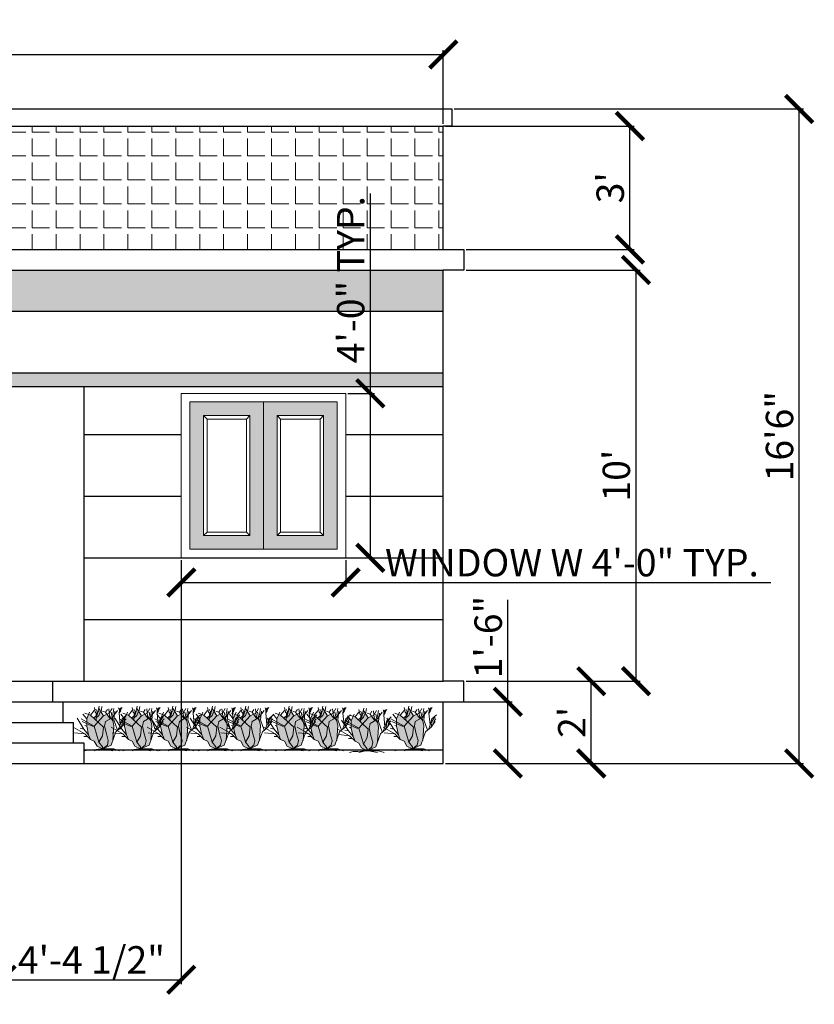
# Model space of a CAD drawing. Units: inches. Extents: x 21865 to 22885, y 36660 to 37408.
# Tile 6 of 6: x 22653 to 22885, y 36873 to 37161. Entities that reach past the tile are written whole.
import ezdxf

# ---------------------------------------------------------------- set-up
doc = ezdxf.new("R2010")
doc.units = ezdxf.units.IN
for name, color, linetype, lineweight in [('A-ANNO-DIMS', 2, 'Continuous', 18), ('A-ELEV', 7, 'Continuous', 30), ('A-ELEV-GLAZ', 4, 'Continuous', 18), ('A-ELEV-ROOF', 7, 'Continuous', 25), ('A-ELEV-ROOF-PATT', 8, 'Continuous', 13), ('L-PLNT', 94, 'Continuous', 13)]:
    doc.layers.add(name, color=color, linetype=linetype, lineweight=lineweight)
for name, color, linetype, lineweight, true_color in [('A-ELEV-TRIM-PATT', 51, 'Continuous', 13, 0xf7f281), ('A-ELEV-WALL-PATT', 251, 'Continuous', 13, 0x636466), ('L-PLNT-PATT', 114, 'Continuous', 13, 0x139b48)]:
    doc.layers.add(name, color=color, linetype=linetype, lineweight=lineweight, true_color=true_color)
doc.styles.get("Standard").update_dxf_attribs({"font": 'arial.ttf'})
doc.dimstyles.new('ISO-25', dxfattribs={"dimtxt": 8, "dimasz": 8, "dimexe": 1.25, "dimexo": 0.625, "dimtad": 1, "dimlunit": 3, "dimtxsty": 'Standard', "dimblk": 'ARCHTICK', "dimcen": 2.5, "dimclrd": 4, "dimclre": 5, "dimclrt": 1, "dimadec": 0, "dimazin": 0, "dimtfac": 1, "dimtmove": 0, "dimatfit": 3, "dimfxl": 1, "dimarcsym": 0})

# ---------------------------------------------------------------- blocks, each defined once
blk = doc.blocks.new('*U12')
for p, q in [((-14.88, 18.24), (-12.96, 20.64)), ((-12.471, 19.775), (-12.898, 22.044)), ((-11.28, 19.619), (-12.104, 21.184)), ((-11.921, 18.836), (-10.64, 20.401)), ((-11.433, 18.289), (-10.457, 22.749)), ((-8.16, 17.76), (-10.56, 21.6)), ((-9.48, 19.775), (-8.992, 22.592)), ((-7.2, 19.68), (-8.64, 20.16)), ((-7.2, 19.68), (-6.24, 21.12)), ((-5.086, 17.741), (-5.513, 21.34)), ((-5.28, 19.2), (-3.84, 21.6)), ((-3.84, 16.8), (-0.96, 20.64)), ((-3.377, 18.602), (-2.888, 21.575)), ((-2.88, 15.84), (-2.4, 20.16)), ((-0.508, 21.888), (-0.081, 20.558)), ((-0.203, 19.149), (0.102, 21.34)), ((-0.142, 19.384), (0.59, 20.401)), ((-0.02, 20.01), (0.896, 21.105)), ((0.041, 20.714), (1.384, 22.044)), ((0.102, 21.34), (0.835, 21.888)), ((-18.24, 11.04), (-21.755, 16.655)), ((-12.96, 12.48), (-19.68, 16.32)), ((-16.8, 16.32), (-18.72, 18.72)), ((-14.88, 18.24), (-17.76, 19.2)), ((-16.8, 16.32), (-15.36, 19.68)), ((-16.8, 12.48), (-16.8, 16.32)), ((-8.16, 12), (-14.88, 18.24)), ((-13.325, 16.724), (-11.433, 18.289)), ((-12.96, 12.48), (-8.16, 17.76)), ((-11.677, 19.071), (-12.471, 19.775)), ((-12.043, 15.628), (-11.921, 18.836)), ((-11.982, 16.802), (-10.579, 18.054)), ((-10.579, 18.054), (-9.846, 19.697)), ((-8.16, 17.76), (-5.28, 19.2)), ((-4.8, 16.32), (-7.2, 19.68)), ((-7.2, 14.88), (-3.84, 16.8)), ((-3.377, 15.315), (-5.086, 17.819)), ((-2.88, 12.96), (-4.32, 19.68)), ((-2.766, 16.802), (-3.377, 18.602)), ((-0.96, 10.56), (-2.88, 15.84)), ((0.346, 13.203), (-0.203, 19.149)), ((0.346, 13.203), (1.323, 16.254)), ((0.96, 12), (1.44, 15.36)), ((1.323, 16.254), (3.642, 18.289)), ((1.44, 15.36), (2.88, 17.28)), ((1.92, 13.44), (2.4, 15.36)), ((2.4, 15.36), (3.36, 16.32)), ((-17.76, 8.64), (-23.663, 11.961)), ((-18.24, 11.04), (-20.16, 11.52)), ((-13.92, 12.48), (-19.2, 14.88)), ((-15.84, 8.16), (-18.24, 11.04)), ((-16.8, 12.48), (-17.76, 12.96)), ((-15.84, 8.16), (-16.8, 12.48)), ((-12.96, 12.48), (-13.92, 12.48)), ((-10.56, 4.32), (-12.96, 12.48)), ((-8.64, 7.68), (-8.16, 12)), ((-7.68, 12.48), (-7.2, 14.88)), ((-6.72, 8.64), (-7.68, 12.48)), ((-3.36, 5.28), (-2.88, 12.96)), ((-1.92, 9.6), (0.96, 12)), ((-0.48, 10.8), (0.346, 13.203)), ((0.96, 12), (2.88, 14.88)), ((-17.76, 8.64), (-23.128, 9.222)), ((-16.32, 7.2), (-18.24, 7.2)), ((-14.88, 5.76), (-17.76, 8.64)), ((-14.88, 5.76), (-15.84, 8.16)), ((-12.96, 4.8), (-14.88, 5.76)), ((-10.56, 4.32), (-8.64, 7.68)), ((-5.76, 5.28), (-6.72, 8.64)), ((-6.24, 2.88), (-5.76, 5.28)), ((-4.32, 2.88), (-1.92, 9.6)), ((-15.84, 0.48), (-17.76, 0)), ((-13.44, 0.48), (-15.84, 0.48)), ((-9.6, 0.96), (-13.44, 0.48)), ((-11.52, 2.4), (-12.96, 4.8)), ((-9.6, 0.96), (-12.96, 0)), ((-8.64, 0.96), (-11.52, 2.4)), ((-8.64, 1.92), (-10.56, 4.32)), ((-9.6, 0.96), (-7.68, 0.96)), ((-8.64, 0.96), (-4.32, 2.88)), ((-8.64, 0.96), (-6.24, 2.88)), ((-8.64, 0.96), (-8.64, 1.92)), ((-8.64, 0.96), (-2.88, 0.96)), ((-7.68, 0.96), (-6.24, 0.48)), ((-6.24, 0.48), (-3.36, 0)), ((-2.88, 0.96), (0, 0))]:
    blk.add_line(p, q)
blk = doc.blocks.new('_ArchTick')
at = {"color": 0, "linetype": 'ByBlock', "const_width": 0.15}
blk.add_lwpolyline([(-0.5, -0.5), (0.5, 0.5)], dxfattribs=at)
blk = doc.blocks.new('*D14')
at = {"layer": 'A-ANNO-DIMS', "color": 0, "lineweight": -2, "transparency": 16777216}
for p, q in [((22416.69, 37130.12), (22416.69, 37151.63)), ((22416.69, 37150.38), (22776.69, 37150.38)), ((22776.69, 37130.12), (22776.69, 37151.63))]:
    blk.add_line(p, q, dxfattribs=at)
at = {"layer": 'Defpoints', "color": 0, "transparency": 16777216}
for p in [(22776.69, 37150.38), (22416.69, 37129.5), (22776.69, 37129.5)]:
    blk.add_point(p, dxfattribs=at)
at = {"layer": 'A-ANNO-DIMS', "color": 0, "lineweight": -2, "transparency": 16777216, "xscale": 8, "yscale": 8, "zscale": 8, "rotation": 180}
blk.add_blockref('_ArchTick', (22416.69, 37150.38), dxfattribs=at)
at = {"layer": 'A-ANNO-DIMS', "color": 0, "lineweight": -2, "transparency": 16777216, "xscale": 8, "yscale": 8, "zscale": 8}
blk.add_blockref('_ArchTick', (22776.69, 37150.38), dxfattribs=at)
at = {"layer": 'A-ANNO-DIMS', "color": 0, "transparency": 16777216, "insert": (22596.69, 37155.1), "char_height": 8, "attachment_point": 5}
blk.add_mtext("30'", dxfattribs=at)
blk = doc.blocks.new('*D15')
at = {"layer": 'A-ANNO-DIMS', "color": 0, "lineweight": -2, "transparency": 16777216}
for p, q in [((22795.53, 36961.5), (22795.53, 36991.26)), ((22777.32, 36961.5), (22796.78, 36961.5)), ((22795.53, 36943.5), (22795.53, 36961.5)), ((22777.32, 36943.5), (22796.78, 36943.5))]:
    blk.add_line(p, q, dxfattribs=at)
at = {"layer": 'Defpoints', "color": 0, "transparency": 16777216}
for p in [(22776.69, 36961.5), (22795.53, 36961.5), (22776.69, 36943.5)]:
    blk.add_point(p, dxfattribs=at)
at = {"layer": 'A-ANNO-DIMS', "color": 0, "lineweight": -2, "transparency": 16777216, "xscale": 8, "yscale": 8, "zscale": 8}
for p, rotation in [((22795.53, 36961.5), 90), ((22795.53, 36943.5), 270)]:
    blk.add_blockref('_ArchTick', p, dxfattribs=dict(at, rotation=rotation))
at = {"layer": 'A-ANNO-DIMS', "color": 0, "transparency": 16777216, "insert": (22790.82, 36980.38), "char_height": 8, "attachment_point": 5, "rotation": 90}
blk.add_mtext('1\'-6"', dxfattribs=at)
blk = doc.blocks.new('*D16')
at = {"layer": 'A-ANNO-DIMS', "color": 0, "lineweight": -2, "transparency": 16777216}
for p, q in [((22783.32, 36967.5), (22821.13, 36967.5)), ((22819.88, 36943.5), (22819.88, 36967.5)), ((22777.32, 36943.5), (22821.13, 36943.5))]:
    blk.add_line(p, q, dxfattribs=at)
at = {"layer": 'Defpoints', "color": 0, "transparency": 16777216}
for p in [(22782.69, 36967.5), (22819.88, 36967.5), (22776.69, 36943.5)]:
    blk.add_point(p, dxfattribs=at)
at = {"layer": 'A-ANNO-DIMS', "color": 0, "lineweight": -2, "transparency": 16777216, "xscale": 8, "yscale": 8, "zscale": 8}
for p, rotation in [((22819.88, 36967.5), 90), ((22819.88, 36943.5), 270)]:
    blk.add_blockref('_ArchTick', p, dxfattribs=dict(at, rotation=rotation))
at = {"layer": 'A-ANNO-DIMS', "color": 0, "transparency": 16777216, "insert": (22815.24, 36955.5), "char_height": 8, "attachment_point": 5, "rotation": 90}
blk.add_mtext("2'", dxfattribs=at)
blk = doc.blocks.new('*D17')
at = {"layer": 'A-ANNO-DIMS', "color": 0, "lineweight": -2, "transparency": 16777216}
for p, q in [((22779.82, 37134.5), (22881.84, 37134.5)), ((22880.59, 36943.5), (22880.59, 37134.5)), ((22777.32, 36943.5), (22881.84, 36943.5))]:
    blk.add_line(p, q, dxfattribs=at)
at = {"layer": 'Defpoints', "color": 0, "transparency": 16777216}
for p in [(22779.19, 37134.5), (22880.59, 37134.5), (22776.69, 36943.5)]:
    blk.add_point(p, dxfattribs=at)
at = {"layer": 'A-ANNO-DIMS', "color": 0, "lineweight": -2, "transparency": 16777216, "xscale": 8, "yscale": 8, "zscale": 8}
for p, rotation in [((22880.59, 37134.5), 90), ((22880.59, 36943.5), 270)]:
    blk.add_blockref('_ArchTick', p, dxfattribs=dict(at, rotation=rotation))
at = {"layer": 'A-ANNO-DIMS', "color": 0, "transparency": 16777216, "insert": (22875.89, 37039), "char_height": 8, "attachment_point": 5, "rotation": 90}
blk.add_mtext('16\'6"', dxfattribs=at)
blk = doc.blocks.new('*D18')
at = {"layer": 'A-ANNO-DIMS', "color": 0, "lineweight": -2, "transparency": 16777216}
for p, q in [((22783.32, 37087.5), (22834.21, 37087.5)), ((22832.96, 36967.5), (22832.96, 37087.5)), ((22783.32, 36967.5), (22834.21, 36967.5))]:
    blk.add_line(p, q, dxfattribs=at)
at = {"layer": 'Defpoints', "color": 0, "transparency": 16777216}
for p in [(22782.69, 37087.5), (22832.96, 37087.5), (22782.69, 36967.5)]:
    blk.add_point(p, dxfattribs=at)
at = {"layer": 'A-ANNO-DIMS', "color": 0, "lineweight": -2, "transparency": 16777216, "xscale": 8, "yscale": 8, "zscale": 8}
for p, rotation in [((22832.96, 37087.5), 90), ((22832.96, 36967.5), 270)]:
    blk.add_blockref('_ArchTick', p, dxfattribs=dict(at, rotation=rotation))
at = {"layer": 'A-ANNO-DIMS', "color": 0, "transparency": 16777216, "insert": (22828.25, 37027.5), "char_height": 8, "attachment_point": 5, "rotation": 90}
blk.add_mtext("10'", dxfattribs=at)
blk = doc.blocks.new('*D19')
at = {"layer": 'A-ANNO-DIMS', "color": 0, "lineweight": -2, "transparency": 16777216}
for p, q in [((22777.32, 37129.5), (22832.42, 37129.5)), ((22831.17, 37093.5), (22831.17, 37129.5)), ((22783.32, 37093.5), (22832.42, 37093.5))]:
    blk.add_line(p, q, dxfattribs=at)
at = {"layer": 'Defpoints', "color": 0, "transparency": 16777216}
for p in [(22776.69, 37129.5), (22831.17, 37129.5), (22782.69, 37093.5)]:
    blk.add_point(p, dxfattribs=at)
at = {"layer": 'A-ANNO-DIMS', "color": 0, "lineweight": -2, "transparency": 16777216, "xscale": 8, "yscale": 8, "zscale": 8}
for p, rotation in [((22831.17, 37129.5), 90), ((22831.17, 37093.5), 270)]:
    blk.add_blockref('_ArchTick', p, dxfattribs=dict(at, rotation=rotation))
at = {"layer": 'A-ANNO-DIMS', "color": 0, "transparency": 16777216, "insert": (22826.46, 37111.5), "char_height": 8, "attachment_point": 5, "rotation": 90}
blk.add_mtext("3'", dxfattribs=at)
blk = doc.blocks.new('WIN-48-ELEV-CASING')
for p, q in [((0, 48), (0, 0)), ((0, 48), (48, 48)), ((48, 48), (48, 0)), ((0, 0), (48, 0))]:
    blk.add_line(p, q)
blk = doc.blocks.new('*D40')
at = {"layer": 'A-ANNO-DIMS', "color": 5, "lineweight": -2, "transparency": 16777216}
for p, q in [((22700.19, 37002.87), (22700.19, 36995.05)), ((22748.19, 37002.87), (22748.19, 36995.05))]:
    blk.add_line(p, q, dxfattribs=at)
at = {"layer": 'A-ANNO-DIMS', "color": 4, "lineweight": -2, "transparency": 16777216}
for p, q in [((22700.19, 36996.3), (22748.19, 36996.3)), ((22748.19, 36996.3), (22872.33, 36996.3))]:
    blk.add_line(p, q, dxfattribs=at)
at = {"layer": 'Defpoints', "color": 0, "transparency": 16777216}
for p in [(22700.19, 37003.5), (22748.19, 37003.5), (22748.19, 36996.3)]:
    blk.add_point(p, dxfattribs=at)
at = {"layer": 'A-ANNO-DIMS', "color": 4, "lineweight": -2, "transparency": 16777216, "xscale": 8, "yscale": 8, "zscale": 8, "rotation": 180}
blk.add_blockref('_ArchTick', (22700.19, 36996.3), dxfattribs=at)
at = {"layer": 'A-ANNO-DIMS', "color": 4, "lineweight": -2, "transparency": 16777216, "xscale": 8, "yscale": 8, "zscale": 8}
blk.add_blockref('_ArchTick', (22748.19, 36996.3), dxfattribs=at)
at = {"layer": 'A-ANNO-DIMS', "color": 1, "transparency": 16777216, "insert": (22814.26, 37001.06), "char_height": 8, "attachment_point": 5}
blk.add_mtext('WINDOW W 4\'-0" TYP.', dxfattribs=at)
blk = doc.blocks.new('*D41')
at = {"layer": 'A-ANNO-DIMS', "color": 4, "lineweight": -2, "transparency": 16777216}
for p, q in [((22755.39, 37051.5), (22755.39, 37109.83)), ((22755.39, 37003.5), (22755.39, 37051.5))]:
    blk.add_line(p, q, dxfattribs=at)
at = {"layer": 'A-ANNO-DIMS', "color": 5, "lineweight": -2, "transparency": 16777216}
for p, q in [((22748.82, 37051.5), (22756.64, 37051.5)), ((22748.82, 37003.5), (22756.64, 37003.5))]:
    blk.add_line(p, q, dxfattribs=at)
at = {"layer": 'Defpoints', "color": 0, "transparency": 16777216}
for p in [(22748.19, 37051.5), (22755.39, 37051.5), (22748.19, 37003.5)]:
    blk.add_point(p, dxfattribs=at)
at = {"layer": 'A-ANNO-DIMS', "color": 4, "lineweight": -2, "transparency": 16777216, "xscale": 8, "yscale": 8, "zscale": 8}
for p, rotation in [((22755.39, 37051.5), 90), ((22755.39, 37003.5), 270)]:
    blk.add_blockref('_ArchTick', p, dxfattribs=dict(at, rotation=rotation))
at = {"layer": 'A-ANNO-DIMS', "color": 1, "transparency": 16777216, "insert": (22750.68, 37084.67), "char_height": 8, "attachment_point": 5, "rotation": 90}
blk.add_mtext('4\'-0" TYP.', dxfattribs=at)
blk = doc.blocks.new('*D63')
at = {"layer": 'A-ANNO-DIMS', "color": 5, "lineweight": -2, "transparency": 16777216}
for p, q in [((22700.19, 37002.87), (22700.19, 36879.13)), ((22647.69, 36966.87), (22647.69, 36879.13))]:
    blk.add_line(p, q, dxfattribs=at)
at = {"layer": 'A-ANNO-DIMS', "color": 4, "lineweight": -2, "transparency": 16777216}
blk.add_line((22647.69, 36880.38), (22700.19, 36880.38), dxfattribs=at)
at = {"layer": 'Defpoints', "color": 0, "transparency": 16777216}
for p in [(22700.19, 37003.5), (22647.69, 36967.5), (22700.19, 36880.38)]:
    blk.add_point(p, dxfattribs=at)
at = {"layer": 'A-ANNO-DIMS', "color": 4, "lineweight": -2, "transparency": 16777216, "xscale": 8, "yscale": 8, "zscale": 8, "rotation": 180}
blk.add_blockref('_ArchTick', (22647.69, 36880.38), dxfattribs=at)
at = {"layer": 'A-ANNO-DIMS', "color": 4, "lineweight": -2, "transparency": 16777216, "xscale": 8, "yscale": 8, "zscale": 8}
blk.add_blockref('_ArchTick', (22700.19, 36880.38), dxfattribs=at)
at = {"layer": 'A-ANNO-DIMS', "color": 1, "transparency": 16777216, "insert": (22673.94, 36885.14), "char_height": 8, "attachment_point": 5}
blk.add_mtext('4\'-4 1/2"', dxfattribs=at)

msp = doc.modelspace()

# ---------------------------------------------------------------- hatches: boundary and pattern name
at = {"layer": 'A-ELEV-ROOF-PATT'}
h = msp.add_hatch(dxfattribs=at)
h.set_pattern_fill('ANGLE', color=256)
h.set_pattern_definition([(0, (486.264, 638.11), (0, 6.985), [5.08, -1.905]), (90, (486.264, 638.11), (-6.985, 4e-16), [5.08, -1.905])])
h.paths.add_polyline_path([(22776.694, 37129.498), (22416.694, 37129.498), (22416.694, 37093.498), (22776.694, 37093.498)])
at = {"layer": 'A-ELEV-TRIM-PATT'}
h = msp.add_hatch(color=256, dxfattribs=at)
h.dxf.hatch_style = 1
h.paths.add_polyline_path([(22724.194, 37048.998), (22702.694, 37048.998), (22702.694, 37005.998), (22724.194, 37005.998)])
h.paths.add_polyline_path([(22706.694, 37044.998), (22720.194, 37044.998), (22720.194, 37009.998), (22706.694, 37009.998)], flags=16)
h.paths.add_polyline_path([(22707.694, 37043.998), (22719.194, 37043.998), (22719.194, 37010.998), (22707.694, 37010.998)], flags=0)
h.paths.add_polyline_path([(22745.694, 37048.998), (22724.194, 37048.998), (22724.194, 37005.998), (22745.694, 37005.998)])
h.paths.add_polyline_path([(22728.194, 37044.998), (22741.694, 37044.998), (22741.694, 37009.998), (22728.194, 37009.998)], flags=16)
h.paths.add_polyline_path([(22729.194, 37043.998), (22740.694, 37043.998), (22740.694, 37010.998), (22729.194, 37010.998)], flags=0)
at = {"layer": 'A-ELEV-WALL-PATT'}
h = msp.add_hatch(color=256, dxfattribs=at)
h.dxf.hatch_style = 1
h.paths.add_polyline_path([(22776.694, 37087.498), (22416.694, 37087.498), (22416.694, 37075.498), (22776.694, 37075.498)])
h.paths.add_polyline_path([(22776.694, 37057.498), (22426.694, 37057.498), (22432.694, 37053.498), (22776.694, 37053.498)])
h.paths.add_polyline_path([(22432.694, 37053.498), (22426.694, 37057.498), (22426.694, 36967.498), (22432.694, 36967.498)])
at = {"layer": 'L-PLNT-PATT'}
h = msp.add_hatch(color=256, dxfattribs=at)
h.dxf.hatch_style = 1
h.paths.add_polyline_path([(22677.499, 36954.067), (22675.88, 36955.571), (22674.762, 36954.341), (22676.131, 36949.688), (22677.226, 36951.604)])
h.paths.add_polyline_path([(22680.51, 36954.615), (22680.221, 36955.967), (22679.737, 36956.676), (22678.047, 36955.71), (22677.773, 36954.341), (22678.321, 36952.151), (22678.868, 36950.235), (22678.594, 36948.866), (22677.226, 36947.771), (22679.689, 36948.866), (22680.249, 36950.434)])
h.paths.add_polyline_path([(22678.321, 36952.151), (22677.773, 36954.341), (22678.047, 36955.71), (22679.435, 36956.503), (22678.479, 36957.842), (22677.499, 36957.352), (22675.88, 36955.571), (22677.499, 36954.067), (22677.226, 36951.604), (22676.131, 36949.688), (22677.226, 36948.319), (22677.226, 36947.771), (22678.594, 36948.866), (22678.868, 36950.235)])
h.paths.add_polyline_path([(22674.762, 36954.341), (22674.215, 36954.341), (22672.572, 36955.088), (22672.572, 36954.341), (22673.12, 36951.877), (22673.667, 36950.509), (22674.762, 36949.961), (22675.583, 36948.593), (22677.226, 36947.771), (22677.226, 36948.319), (22676.131, 36949.688)])
h.paths.add_polyline_path([(22675.88, 36955.571), (22673.667, 36957.626), (22673.12, 36957.808), (22672.572, 36956.531), (22672.572, 36955.592), (22674.762, 36954.341)])
h.paths.add_polyline_path([(22677.499, 36957.352), (22676.068, 36959.642), (22675.633, 36957.654), (22675.333, 36957.406), (22675.284, 36956.124), (22675.88, 36955.571)])
h.paths.add_polyline_path([(22675.333, 36957.406), (22674.577, 36956.781), (22675.284, 36956.124)], flags=17)
h.paths.add_polyline_path([(22672.572, 36955.592), (22672.572, 36955.088), (22674.215, 36954.341), (22674.762, 36954.341)], flags=17)
h = msp.add_hatch(color=256, dxfattribs=at)
h.dxf.hatch_style = 1
h.paths.add_polyline_path([(22688.566, 36954.067), (22686.947, 36955.571), (22685.829, 36954.341), (22687.198, 36949.688), (22688.293, 36951.604)])
h.paths.add_polyline_path([(22691.577, 36954.615), (22691.288, 36955.967), (22690.804, 36956.676), (22689.114, 36955.71), (22688.84, 36954.341), (22689.388, 36952.151), (22689.935, 36950.235), (22689.661, 36948.866), (22688.293, 36947.771), (22690.756, 36948.866), (22691.316, 36950.434)])
h.paths.add_polyline_path([(22689.388, 36952.151), (22688.84, 36954.341), (22689.114, 36955.71), (22690.502, 36956.503), (22689.546, 36957.842), (22688.566, 36957.352), (22686.947, 36955.571), (22688.566, 36954.067), (22688.293, 36951.604), (22687.198, 36949.688), (22688.293, 36948.319), (22688.293, 36947.771), (22689.661, 36948.866), (22689.935, 36950.235)])
h.paths.add_polyline_path([(22685.829, 36954.341), (22685.282, 36954.341), (22683.639, 36955.088), (22683.639, 36954.341), (22684.187, 36951.877), (22684.734, 36950.509), (22685.829, 36949.961), (22686.65, 36948.593), (22688.293, 36947.771), (22688.293, 36948.319), (22687.198, 36949.688)])
h.paths.add_polyline_path([(22686.947, 36955.571), (22684.734, 36957.626), (22684.187, 36957.808), (22683.639, 36956.531), (22683.639, 36955.592), (22685.829, 36954.341)])
h.paths.add_polyline_path([(22688.566, 36957.352), (22687.135, 36959.642), (22686.7, 36957.654), (22686.4, 36957.406), (22686.352, 36956.124), (22686.947, 36955.571)])
h.paths.add_polyline_path([(22686.4, 36957.406), (22685.644, 36956.781), (22686.352, 36956.124)], flags=17)
h.paths.add_polyline_path([(22683.639, 36955.592), (22683.639, 36955.088), (22685.282, 36954.341), (22685.829, 36954.341)], flags=17)
h = msp.add_hatch(color=256, dxfattribs=at)
h.dxf.hatch_style = 1
h.paths.add_polyline_path([(22699.065, 36954.067), (22697.445, 36955.571), (22696.327, 36954.341), (22697.696, 36949.688), (22698.791, 36951.604)])
h.paths.add_polyline_path([(22702.076, 36954.615), (22701.786, 36955.967), (22701.302, 36956.676), (22699.612, 36955.71), (22699.338, 36954.341), (22699.886, 36952.151), (22700.433, 36950.235), (22700.16, 36948.866), (22698.791, 36947.771), (22701.254, 36948.866), (22701.814, 36950.434)])
h.paths.add_polyline_path([(22699.886, 36952.151), (22699.338, 36954.341), (22699.612, 36955.71), (22701.001, 36956.503), (22700.044, 36957.842), (22699.065, 36957.352), (22697.445, 36955.571), (22699.065, 36954.067), (22698.791, 36951.604), (22697.696, 36949.688), (22698.791, 36948.319), (22698.791, 36947.771), (22700.16, 36948.866), (22700.433, 36950.235)])
h.paths.add_polyline_path([(22696.327, 36954.341), (22695.78, 36954.341), (22694.137, 36955.088), (22694.137, 36954.341), (22694.685, 36951.877), (22695.232, 36950.509), (22696.327, 36949.961), (22697.148, 36948.593), (22698.791, 36947.771), (22698.791, 36948.319), (22697.696, 36949.688)])
h.paths.add_polyline_path([(22697.445, 36955.571), (22695.232, 36957.626), (22694.685, 36957.808), (22694.137, 36956.531), (22694.137, 36955.592), (22696.327, 36954.341)])
h.paths.add_polyline_path([(22699.065, 36957.352), (22697.633, 36959.642), (22697.198, 36957.654), (22696.899, 36957.406), (22696.85, 36956.124), (22697.445, 36955.571)])
h.paths.add_polyline_path([(22696.899, 36957.406), (22696.143, 36956.781), (22696.85, 36956.124)], flags=17)
h.paths.add_polyline_path([(22694.137, 36955.592), (22694.137, 36955.088), (22695.78, 36954.341), (22696.327, 36954.341)], flags=17)
h = msp.add_hatch(color=256, dxfattribs=at)
h.dxf.hatch_style = 1
h.paths.add_polyline_path([(22710.558, 36954.067), (22708.939, 36955.571), (22707.821, 36954.341), (22709.19, 36949.688), (22710.285, 36951.604)])
h.paths.add_polyline_path([(22713.569, 36954.615), (22713.28, 36955.967), (22712.796, 36956.676), (22711.106, 36955.71), (22710.832, 36954.341), (22711.379, 36952.151), (22711.927, 36950.235), (22711.653, 36948.866), (22710.285, 36947.771), (22712.748, 36948.866), (22713.308, 36950.434)])
h.paths.add_polyline_path([(22711.379, 36952.151), (22710.832, 36954.341), (22711.106, 36955.71), (22712.494, 36956.503), (22711.538, 36957.842), (22710.558, 36957.352), (22708.939, 36955.571), (22710.558, 36954.067), (22710.285, 36951.604), (22709.19, 36949.688), (22710.285, 36948.319), (22710.285, 36947.771), (22711.653, 36948.866), (22711.927, 36950.235)])
h.paths.add_polyline_path([(22707.821, 36954.341), (22707.273, 36954.341), (22705.631, 36955.088), (22705.631, 36954.341), (22706.179, 36951.877), (22706.726, 36950.509), (22707.821, 36949.961), (22708.642, 36948.593), (22710.285, 36947.771), (22710.285, 36948.319), (22709.19, 36949.688)])
h.paths.add_polyline_path([(22708.939, 36955.571), (22706.726, 36957.626), (22706.179, 36957.808), (22705.631, 36956.531), (22705.631, 36955.592), (22707.821, 36954.341)])
h.paths.add_polyline_path([(22710.558, 36957.352), (22709.127, 36959.642), (22708.692, 36957.654), (22708.392, 36957.406), (22708.343, 36956.124), (22708.939, 36955.571)])
h.paths.add_polyline_path([(22708.392, 36957.406), (22707.636, 36956.781), (22708.343, 36956.124)], flags=17)
h.paths.add_polyline_path([(22705.631, 36955.592), (22705.631, 36955.088), (22707.273, 36954.341), (22707.821, 36954.341)], flags=17)
h = msp.add_hatch(color=256, dxfattribs=at)
h.dxf.hatch_style = 1
h.paths.add_polyline_path([(22720.294, 36954.067), (22718.675, 36955.571), (22717.556, 36954.341), (22718.925, 36949.688), (22720.02, 36951.604)])
h.paths.add_polyline_path([(22723.305, 36954.615), (22723.015, 36955.967), (22722.532, 36956.676), (22720.841, 36955.71), (22720.568, 36954.341), (22721.115, 36952.151), (22721.662, 36950.235), (22721.389, 36948.866), (22720.02, 36947.771), (22722.484, 36948.866), (22723.044, 36950.434)])
h.paths.add_polyline_path([(22721.115, 36952.151), (22720.568, 36954.341), (22720.841, 36955.71), (22722.23, 36956.503), (22721.274, 36957.842), (22720.294, 36957.352), (22718.675, 36955.571), (22720.294, 36954.067), (22720.02, 36951.604), (22718.925, 36949.688), (22720.02, 36948.319), (22720.02, 36947.771), (22721.389, 36948.866), (22721.662, 36950.235)])
h.paths.add_polyline_path([(22717.556, 36954.341), (22717.009, 36954.341), (22715.367, 36955.088), (22715.367, 36954.341), (22715.914, 36951.877), (22716.462, 36950.509), (22717.556, 36949.961), (22718.378, 36948.593), (22720.02, 36947.771), (22720.02, 36948.319), (22718.925, 36949.688)])
h.paths.add_polyline_path([(22718.675, 36955.571), (22716.462, 36957.626), (22715.914, 36957.808), (22715.367, 36956.531), (22715.367, 36955.592), (22717.556, 36954.341)])
h.paths.add_polyline_path([(22720.294, 36957.352), (22718.862, 36959.642), (22718.427, 36957.654), (22718.128, 36957.406), (22718.079, 36956.124), (22718.675, 36955.571)])
h.paths.add_polyline_path([(22718.128, 36957.406), (22717.372, 36956.781), (22718.079, 36956.124)], flags=17)
h.paths.add_polyline_path([(22715.367, 36955.592), (22715.367, 36955.088), (22717.009, 36954.341), (22717.556, 36954.341)], flags=17)
h = msp.add_hatch(color=256, dxfattribs=at)
h.dxf.hatch_style = 1
h.paths.add_polyline_path([(22733.032, 36954.067), (22731.412, 36955.571), (22730.294, 36954.341), (22731.663, 36949.688), (22732.758, 36951.604)])
h.paths.add_polyline_path([(22736.043, 36954.615), (22735.753, 36955.967), (22735.269, 36956.676), (22733.579, 36955.71), (22733.305, 36954.341), (22733.853, 36952.151), (22734.4, 36950.235), (22734.127, 36948.866), (22732.758, 36947.771), (22735.221, 36948.866), (22735.781, 36950.434)])
h.paths.add_polyline_path([(22733.853, 36952.151), (22733.305, 36954.341), (22733.579, 36955.71), (22734.968, 36956.503), (22734.011, 36957.842), (22733.032, 36957.352), (22731.412, 36955.571), (22733.032, 36954.067), (22732.758, 36951.604), (22731.663, 36949.688), (22732.758, 36948.319), (22732.758, 36947.771), (22734.127, 36948.866), (22734.4, 36950.235)])
h.paths.add_polyline_path([(22730.294, 36954.341), (22729.747, 36954.341), (22728.104, 36955.088), (22728.104, 36954.341), (22728.652, 36951.877), (22729.199, 36950.509), (22730.294, 36949.961), (22731.115, 36948.593), (22732.758, 36947.771), (22732.758, 36948.319), (22731.663, 36949.688)])
h.paths.add_polyline_path([(22731.412, 36955.571), (22729.199, 36957.626), (22728.652, 36957.808), (22728.104, 36956.531), (22728.104, 36955.592), (22730.294, 36954.341)])
h.paths.add_polyline_path([(22733.032, 36957.352), (22731.6, 36959.642), (22731.165, 36957.654), (22730.866, 36957.406), (22730.817, 36956.124), (22731.412, 36955.571)])
h.paths.add_polyline_path([(22730.866, 36957.406), (22730.11, 36956.781), (22730.817, 36956.124)], flags=17)
h.paths.add_polyline_path([(22728.104, 36955.592), (22728.104, 36955.088), (22729.747, 36954.341), (22730.294, 36954.341)], flags=17)
h = msp.add_hatch(color=256, dxfattribs=at)
h.dxf.hatch_style = 1
h.paths.add_polyline_path([(22742.857, 36954.067), (22741.238, 36955.571), (22740.12, 36954.341), (22741.489, 36949.688), (22742.584, 36951.604)])
h.paths.add_polyline_path([(22745.869, 36954.615), (22745.579, 36955.967), (22745.095, 36956.676), (22743.405, 36955.71), (22743.131, 36954.341), (22743.679, 36952.151), (22744.226, 36950.235), (22743.952, 36948.866), (22742.584, 36947.771), (22745.047, 36948.866), (22745.607, 36950.434)])
h.paths.add_polyline_path([(22743.679, 36952.151), (22743.131, 36954.341), (22743.405, 36955.71), (22744.793, 36956.503), (22743.837, 36957.842), (22742.857, 36957.352), (22741.238, 36955.571), (22742.857, 36954.067), (22742.584, 36951.604), (22741.489, 36949.688), (22742.584, 36948.319), (22742.584, 36947.771), (22743.952, 36948.866), (22744.226, 36950.235)])
h.paths.add_polyline_path([(22740.12, 36954.341), (22739.573, 36954.341), (22737.93, 36955.088), (22737.93, 36954.341), (22738.478, 36951.877), (22739.025, 36950.509), (22740.12, 36949.961), (22740.941, 36948.593), (22742.584, 36947.771), (22742.584, 36948.319), (22741.489, 36949.688)])
h.paths.add_polyline_path([(22741.238, 36955.571), (22739.025, 36957.626), (22738.478, 36957.808), (22737.93, 36956.531), (22737.93, 36955.592), (22740.12, 36954.341)])
h.paths.add_polyline_path([(22742.857, 36957.352), (22741.426, 36959.642), (22740.991, 36957.654), (22740.691, 36957.406), (22740.643, 36956.124), (22741.238, 36955.571)])
h.paths.add_polyline_path([(22740.691, 36957.406), (22739.935, 36956.781), (22740.643, 36956.124)], flags=17)
h.paths.add_polyline_path([(22737.93, 36955.592), (22737.93, 36955.088), (22739.573, 36954.341), (22740.12, 36954.341)], flags=17)
h = msp.add_hatch(color=256, dxfattribs=at)
h.dxf.hatch_style = 1
h.paths.add_polyline_path([(22754.752, 36953.52), (22753.133, 36955.023), (22752.015, 36953.794), (22753.383, 36949.14), (22754.478, 36951.056)])
h.paths.add_polyline_path([(22757.763, 36954.067), (22757.473, 36955.42), (22756.99, 36956.128), (22755.299, 36955.162), (22755.026, 36953.794), (22755.573, 36951.604), (22756.121, 36949.688), (22755.847, 36948.319), (22754.478, 36947.224), (22756.942, 36948.319), (22757.502, 36949.887)])
h.paths.add_polyline_path([(22755.573, 36951.604), (22755.026, 36953.794), (22755.299, 36955.162), (22756.688, 36955.956), (22755.732, 36957.294), (22754.752, 36956.805), (22753.133, 36955.023), (22754.752, 36953.52), (22754.478, 36951.056), (22753.383, 36949.14), (22754.478, 36947.771), (22754.478, 36947.224), (22755.847, 36948.319), (22756.121, 36949.688)])
h.paths.add_polyline_path([(22752.015, 36953.794), (22751.467, 36953.794), (22749.825, 36954.54), (22749.825, 36953.794), (22750.372, 36951.33), (22750.92, 36949.961), (22752.015, 36949.414), (22752.836, 36948.045), (22754.478, 36947.224), (22754.478, 36947.771), (22753.383, 36949.14)])
h.paths.add_polyline_path([(22753.133, 36955.023), (22750.92, 36957.078), (22750.372, 36957.261), (22749.825, 36955.983), (22749.825, 36955.045), (22752.015, 36953.794)])
h.paths.add_polyline_path([(22754.752, 36956.805), (22753.321, 36959.095), (22752.886, 36957.106), (22752.586, 36956.859), (22752.537, 36955.576), (22753.133, 36955.023)])
h.paths.add_polyline_path([(22752.586, 36956.859), (22751.83, 36956.233), (22752.537, 36955.576)], flags=17)
h.paths.add_polyline_path([(22749.825, 36955.045), (22749.825, 36954.54), (22751.467, 36953.794), (22752.015, 36953.794)], flags=17)
h = msp.add_hatch(color=256, dxfattribs=at)
h.dxf.hatch_style = 1
h.paths.add_polyline_path([(22767.97, 36954.067), (22766.351, 36955.571), (22765.233, 36954.341), (22766.602, 36949.688), (22767.696, 36951.604)])
h.paths.add_polyline_path([(22770.981, 36954.615), (22770.691, 36955.967), (22770.208, 36956.676), (22768.518, 36955.71), (22768.244, 36954.341), (22768.791, 36952.151), (22769.339, 36950.235), (22769.065, 36948.866), (22767.696, 36947.771), (22770.16, 36948.866), (22770.72, 36950.434)])
h.paths.add_polyline_path([(22768.791, 36952.151), (22768.244, 36954.341), (22768.518, 36955.71), (22769.906, 36956.503), (22768.95, 36957.842), (22767.97, 36957.352), (22766.351, 36955.571), (22767.97, 36954.067), (22767.696, 36951.604), (22766.602, 36949.688), (22767.696, 36948.319), (22767.696, 36947.771), (22769.065, 36948.866), (22769.339, 36950.235)])
h.paths.add_polyline_path([(22765.233, 36954.341), (22764.685, 36954.341), (22763.043, 36955.088), (22763.043, 36954.341), (22763.59, 36951.877), (22764.138, 36950.509), (22765.233, 36949.961), (22766.054, 36948.593), (22767.696, 36947.771), (22767.696, 36948.319), (22766.602, 36949.688)])
h.paths.add_polyline_path([(22766.351, 36955.571), (22764.138, 36957.626), (22763.59, 36957.808), (22763.043, 36956.531), (22763.043, 36955.592), (22765.233, 36954.341)])
h.paths.add_polyline_path([(22767.97, 36957.352), (22766.539, 36959.642), (22766.104, 36957.654), (22765.804, 36957.406), (22765.755, 36956.124), (22766.351, 36955.571)])
h.paths.add_polyline_path([(22765.804, 36957.406), (22765.048, 36956.781), (22765.755, 36956.124)], flags=17)
h.paths.add_polyline_path([(22763.043, 36955.592), (22763.043, 36955.088), (22764.685, 36954.341), (22765.233, 36954.341)], flags=17)

# ---------------------------------------------------------------- linework, layer by layer
at = {"layer": 'A-ELEV'}
for p, q in [((22776.694, 36967.498), (22776.694, 37087.498)), ((22416.694, 37075.498), (22776.694, 37075.498)), ((22426.694, 37057.498), (22776.694, 37057.498)), ((22432.694, 37053.498), (22776.694, 37053.498)), ((22671.694, 37053.498), (22671.694, 36967.498)), ((22671.694, 37039.498), (22700.194, 37039.498)), ((22748.194, 37039.498), (22776.694, 37039.498)), ((22671.694, 37021.498), (22700.194, 37021.498)), ((22748.194, 37021.498), (22776.694, 37021.498)), ((22671.694, 37003.498), (22776.694, 37003.498)), ((22671.694, 36985.498), (22776.694, 36985.498)), ((22416.694, 36967.498), (22671.694, 36967.498)), ((22662.694, 36961.498), (22662.694, 36967.498)), ((22671.694, 36967.498), (22776.694, 36967.498)), ((22782.694, 36967.498), (22776.694, 36967.498)), ((22782.694, 36961.498), (22782.694, 36967.498)), ((22581.694, 36961.498), (22776.694, 36961.498)), ((22665.694, 36955.498), (22665.694, 36961.498)), ((22776.694, 36943.498), (22776.694, 36961.498)), ((22776.694, 36961.498), (22782.694, 36961.498)), ((22578.694, 36955.498), (22668.694, 36955.498)), ((22668.694, 36949.498), (22668.694, 36955.498)), ((22575.694, 36949.498), (22671.694, 36949.498)), ((22671.694, 36949.498), (22671.694, 36943.498)), ((22671.694, 36947.498), (22776.694, 36947.498)), ((22416.694, 36943.498), (22776.694, 36943.498))]:
    msp.add_line(p, q, dxfattribs=at)
at = {"layer": 'A-ELEV-GLAZ'}
for p, q in [((22702.694, 37048.998), (22702.694, 37005.998)), ((22702.694, 37048.998), (22745.694, 37048.998)), ((22724.194, 37005.998), (22724.194, 37048.998)), ((22745.694, 37048.998), (22745.694, 37005.998)), ((22706.694, 37044.998), (22706.694, 37009.998)), ((22706.694, 37044.998), (22720.194, 37044.998)), ((22707.694, 37043.998), (22706.694, 37044.998)), ((22707.694, 37043.998), (22707.694, 37010.998)), ((22707.694, 37043.998), (22719.194, 37043.998)), ((22719.194, 37043.998), (22720.194, 37044.998)), ((22719.194, 37043.998), (22719.194, 37010.998)), ((22720.194, 37044.998), (22720.194, 37009.998)), ((22728.194, 37044.998), (22728.194, 37009.998)), ((22728.194, 37044.998), (22741.694, 37044.998)), ((22729.194, 37043.998), (22728.194, 37044.998)), ((22729.194, 37043.998), (22729.194, 37010.998)), ((22740.694, 37043.998), (22729.194, 37043.998)), ((22740.694, 37043.998), (22741.694, 37044.998)), ((22740.694, 37043.998), (22740.694, 37010.998)), ((22741.694, 37044.998), (22741.694, 37009.998)), ((22707.694, 37010.998), (22706.694, 37009.998)), ((22706.694, 37009.998), (22720.194, 37009.998)), ((22707.694, 37010.998), (22719.194, 37010.998)), ((22719.194, 37010.998), (22720.194, 37009.998)), ((22729.194, 37010.998), (22728.194, 37009.998)), ((22728.194, 37009.998), (22741.694, 37009.998)), ((22740.694, 37010.998), (22729.194, 37010.998)), ((22740.694, 37010.998), (22741.694, 37009.998)), ((22702.694, 37005.998), (22745.694, 37005.998))]:
    msp.add_line(p, q, dxfattribs=at)
at = {"layer": 'A-ELEV-ROOF'}
for p, q in [((22416.694, 37134.498), (22776.694, 37134.498)), ((22776.694, 37134.498), (22779.194, 37134.498)), ((22779.194, 37134.498), (22779.194, 37129.498)), ((22416.694, 37129.498), (22776.694, 37129.498)), ((22776.694, 37093.498), (22776.694, 37129.498)), ((22779.194, 37129.498), (22776.694, 37129.498)), ((22416.694, 37093.498), (22776.694, 37093.498)), ((22776.694, 37093.498), (22782.694, 37093.498)), ((22782.694, 37093.498), (22782.694, 37087.498)), ((22416.694, 37087.498), (22776.694, 37087.498)), ((22782.694, 37087.498), (22776.694, 37087.498))]:
    msp.add_line(p, q, dxfattribs=at)

# ---------------------------------------------------------------- block references
at = {"layer": 'A-ELEV-GLAZ'}
msp.add_blockref('WIN-48-ELEV-CASING', (22700.194, 37003.498), dxfattribs=at)
at = {"layer": 'L-PLNT', "xscale": 0.57027724310695, "yscale": 0.57027724310695, "zscale": 0.57027724310695}
for p in [(22682.153, 36947.224), (22693.22, 36947.224), (22703.718, 36947.224), (22715.212, 36947.224), (22724.947, 36947.224), (22737.685, 36947.224), (22747.511, 36947.224), (22772.624, 36947.224), (22759.405, 36946.677)]:
    msp.add_blockref('*U12', p, dxfattribs=at)

# ---------------------------------------------------------------- dimensions: what is measured, and where the dimension line sits
at = {"layer": 'A-ANNO-DIMS'}
for base, p1, p2, override, picture, middle in [((22776.694, 37150.383), (22416.694, 37129.498), (22776.694, 37129.498), {"dimclrd": 0, "dimclre": 0, "dimclrt": 0}, '*D14', (22596.694, 37155.095)), ((22700.194, 36880.381), (22647.694, 36967.498), (22700.194, 37003.498), {"dimdec": 1, "dimlfac": 1, "dimrnd": 0, "dimzin": 1, "dimdsep": 46, "dimlunit": 4, "dimfrac": 2}, '*D63', (22673.944, 36885.142))]:
    dim = msp.add_linear_dim(base=base, p1=p1, p2=p2, dimstyle='ISO-25', override=override, dxfattribs=at)
    dim.commit()
    dim.dimension.update_dxf_attribs({"geometry": picture, "text_midpoint": middle})
for base, p1, p2, text, override, picture, middle in [((22880.595, 37134.498), (22776.694, 36943.498), (22779.194, 37134.498), '16\'6"', {"dimclrd": 0, "dimclre": 0, "dimclrt": 0}, '*D17', (22875.885, 37038.998)), ((22755.394, 37051.498), (22748.194, 37003.498), (22748.194, 37051.498), '<> TYP.', {"dimdec": 1, "dimlfac": 1, "dimrnd": 0, "dimzin": 1, "dimdsep": 46, "dimlunit": 4, "dimfrac": 2}, '*D41', (22750.684, 37084.666))]:
    dim = msp.add_linear_dim(base=base, p1=p1, p2=p2, angle=90, text=text, dimstyle='ISO-25', override=override, dxfattribs=at)
    dim.commit()
    dim.dimension.update_dxf_attribs({"geometry": picture, "text_midpoint": middle})
for base, p1, p2, picture, middle in [((22831.17, 37129.498), (22782.694, 37093.498), (22776.694, 37129.498), '*D19', (22826.458, 37111.498)), ((22832.959, 37087.498), (22782.694, 36967.498), (22782.694, 37087.498), '*D18', (22828.25, 37027.498)), ((22795.531, 36961.498), (22776.694, 36943.498), (22776.694, 36961.498), '*D15', (22790.822, 36980.379)), ((22819.879, 36967.498), (22776.694, 36943.498), (22782.694, 36967.498), '*D16', (22815.237, 36955.498))]:
    dim = msp.add_linear_dim(base=base, p1=p1, p2=p2, angle=90, dimstyle='ISO-25', override={"dimclrd": 0, "dimclre": 0, "dimclrt": 0}, dxfattribs=at)
    dim.commit()
    dim.dimension.update_dxf_attribs({"geometry": picture, "text_midpoint": middle})
dim = msp.add_linear_dim(base=(22748.194, 36996.298), p1=(22700.194, 37003.498), p2=(22748.194, 37003.498), text='WINDOW W <> TYP.', dimstyle='ISO-25', override={"dimdec": 1, "dimlfac": 1, "dimrnd": 0, "dimzin": 1, "dimdsep": 46, "dimlunit": 4, "dimfrac": 2}, dxfattribs=at)
dim.commit()
dim.dimension.update_dxf_attribs({"geometry": '*D40', "text_midpoint": (22814.262, 37001.062)})

doc.saveas('drawing.dxf')
